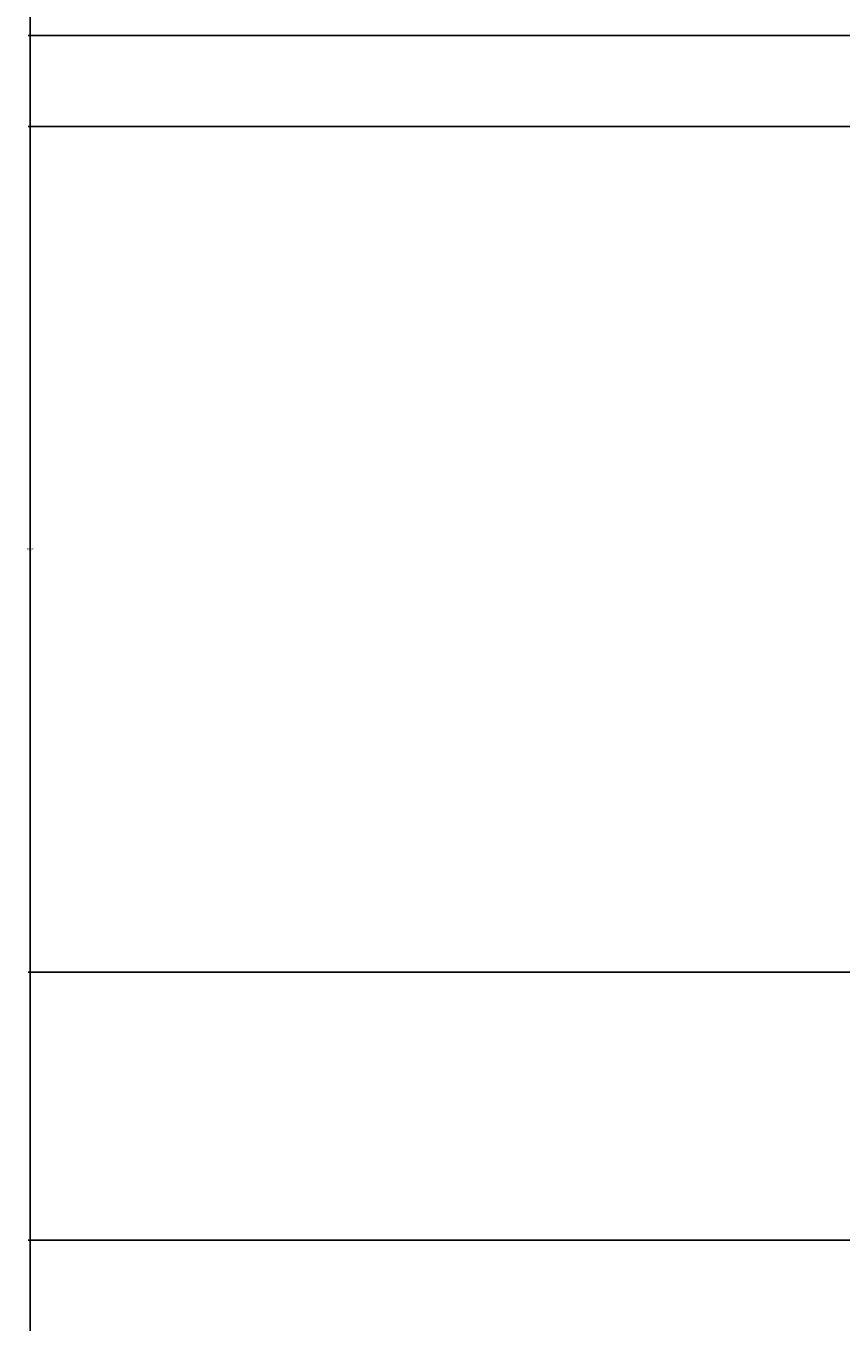
# Model space of a CAD drawing. Units: inches. Extents: x -61 to 1599, y -1316 to 257.
# Tile 56 of 204: x -61 to 12, y -282 to -166. Entities that reach past the tile are written whole.
import ezdxf

# ---------------------------------------------------------------- set-up
doc = ezdxf.new("R2010")
doc.units = ezdxf.units.IN
doc.header["$MEASUREMENT"] = 0
doc.layers.add('A-ANNO-DIMS', color=2, linetype='Continuous', lineweight=18)
doc.styles.get("Standard").update_dxf_attribs({"font": 'arial.ttf'})
doc.dimstyles.get("Standard").update_dxf_attribs({"dimtxt": 0.18, "dimasz": 0.18, "dimexe": 0.18, "dimexo": 0.0625, "dimgap": 0.09, "dimtad": 0, "dimtih": 1, "dimtoh": 1, "dimdec": 0, "dimzin": 0, "dimdsep": 46, "dimlunit": 3, "dimtxsty": 'Standard', "dimcen": 0.09, "dimadec": 0, "dimazin": 0, "dimtfac": 1, "dimtdec": 0, "dimtofl": 0, "dimtmove": 0, "dimatfit": 3, "dimfxl": 1, "dimtolj": 1, "dimtzin": 0, "dimarcsym": 0})

# ---------------------------------------------------------------- blocks, each defined once
blk = doc.blocks.new('*D687')
at = {"layer": 'A-ANNO-DIMS', "color": 0, "lineweight": -2, "transparency": 16777216}
for p, q in [((289.42, 181.68), (-61.08, 181.68)), ((-60.9, 181.5), (-60.9, -528.95)), ((-60.9, -1239.76), (-60.9, -529.32)), ((319.64, -1239.94), (-61.08, -1239.94))]:
    blk.add_line(p, q, dxfattribs=at)
at = {"layer": 'A-ANNO-DIMS', "color": 0, "transparency": 16777216}
for points in [[(-60.93, 181.5), (-60.87, 181.5), (-60.9, 181.68)], [(-60.93, -1239.76), (-60.87, -1239.76), (-60.9, -1239.94)]]:
    blk.add_solid(points, dxfattribs=at)
at = {"layer": 'DEFPOINTS', "color": 0, "transparency": 16777216}
for p in [(289.48, 181.68), (-60.9, -1239.94), (319.7, -1239.94)]:
    blk.add_point(p, dxfattribs=at)
at = {"layer": 'A-ANNO-DIMS', "color": 0, "transparency": 16777216, "insert": (-60.9, -529.13), "char_height": 0.18, "attachment_point": 5}
blk.add_mtext('\\A1;1421.6', dxfattribs=at)
blk = doc.blocks.new('*D691')
at = {"layer": 'A-ANNO-DIMS', "color": 0, "lineweight": -2, "transparency": 16777216}
for p, q in [((14.64, 157.68), (-61.08, 157.68)), ((-60.9, 157.5), (-60.9, -141.64)), ((-60.9, -441.14), (-60.9, -142)), ((14.64, -441.32), (-61.08, -441.32))]:
    blk.add_line(p, q, dxfattribs=at)
at = {"layer": 'A-ANNO-DIMS', "color": 0, "transparency": 16777216}
for points in [[(-60.93, 157.5), (-60.87, 157.5), (-60.9, 157.68)], [(-60.93, -441.14), (-60.87, -441.14), (-60.9, -441.32)]]:
    blk.add_solid(points, dxfattribs=at)
at = {"layer": 'DEFPOINTS', "color": 0, "transparency": 16777216}
for p in [(-60.9, 157.68), (14.7, 157.68), (14.7, -441.32)]:
    blk.add_point(p, dxfattribs=at)
at = {"layer": 'A-ANNO-DIMS', "color": 0, "transparency": 16777216, "insert": (-60.9, -141.82), "char_height": 0.18, "attachment_point": 5}
blk.add_mtext('\\A1;599', dxfattribs=at)
blk = doc.blocks.new('*D699')
at = {"layer": 'A-ANNO-DIMS', "color": 0, "lineweight": -2, "transparency": 16777216}
for p, q in [((835.64, -167.17), (-61.08, -167.17)), ((-60.9, -167.35), (-60.9, -306.73)), ((-60.9, -446.47), (-60.9, -307.09)), ((841.64, -446.65), (-61.08, -446.65))]:
    blk.add_line(p, q, dxfattribs=at)
at = {"layer": 'A-ANNO-DIMS', "color": 0, "transparency": 16777216}
for points in [[(-60.93, -167.35), (-60.87, -167.35), (-60.9, -167.17)], [(-60.93, -446.47), (-60.87, -446.47), (-60.9, -446.65)]]:
    blk.add_solid(points, dxfattribs=at)
at = {"layer": 'DEFPOINTS', "color": 0, "transparency": 16777216}
for p in [(835.7, -167.17), (-60.9, -446.65), (841.7, -446.65)]:
    blk.add_point(p, dxfattribs=at)
at = {"layer": 'A-ANNO-DIMS', "color": 0, "transparency": 16777216, "insert": (-60.9, -306.91), "char_height": 0.18, "attachment_point": 5}
blk.add_mtext('\\A1;279.5', dxfattribs=at)
blk = doc.blocks.new('*D706')
at = {"layer": 'A-ANNO-DIMS', "color": 0, "lineweight": -2, "transparency": 16777216}
for p, q in [((78.64, -175.32), (-61.08, -175.32)), ((-60.9, -175.5), (-60.9, -212.98)), ((-60.9, -250.81), (-60.9, -213.34)), ((78.64, -250.99), (-61.08, -250.99))]:
    blk.add_line(p, q, dxfattribs=at)
at = {"layer": 'A-ANNO-DIMS', "color": 0, "transparency": 16777216}
for points in [[(-60.93, -175.5), (-60.87, -175.5), (-60.9, -175.32)], [(-60.93, -250.81), (-60.87, -250.81), (-60.9, -250.99)]]:
    blk.add_solid(points, dxfattribs=at)
at = {"layer": 'DEFPOINTS', "color": 0, "transparency": 16777216}
for p in [(-60.9, -175.32), (78.7, -175.32), (78.7, -250.99)]:
    blk.add_point(p, dxfattribs=at)
at = {"layer": 'A-ANNO-DIMS', "color": 0, "transparency": 16777216, "insert": (-60.9, -213.16), "char_height": 0.18, "attachment_point": 5}
blk.add_mtext('\\A1;75.67', dxfattribs=at)
blk = doc.blocks.new('*D707')
at = {"layer": 'A-ANNO-DIMS', "color": 0, "lineweight": -2, "transparency": 16777216}
for p, q in [((78.64, -274.99), (-61.08, -274.99)), ((-60.9, -275.17), (-60.9, -308.47)), ((-60.9, -342.14), (-60.9, -308.84)), ((78.64, -342.32), (-61.08, -342.32))]:
    blk.add_line(p, q, dxfattribs=at)
at = {"layer": 'A-ANNO-DIMS', "color": 0, "transparency": 16777216}
for points in [[(-60.93, -275.17), (-60.87, -275.17), (-60.9, -274.99)], [(-60.93, -342.14), (-60.87, -342.14), (-60.9, -342.32)]]:
    blk.add_solid(points, dxfattribs=at)
at = {"layer": 'DEFPOINTS', "color": 0, "transparency": 16777216}
for p in [(78.7, -274.99), (-60.9, -342.32), (78.7, -342.32)]:
    blk.add_point(p, dxfattribs=at)
at = {"layer": 'A-ANNO-DIMS', "color": 0, "transparency": 16777216, "insert": (-60.9, -308.66), "char_height": 0.18, "attachment_point": 5}
blk.add_mtext('\\A1;67.33', dxfattribs=at)

msp = doc.modelspace()

# ---------------------------------------------------------------- dimensions: what is measured, and where the dimension line sits
at = {"layer": 'A-ANNO-DIMS'}
for base, p1, p2, override, picture, middle in [((-60.8972, -1239.9446), (289.4807, 181.6771), (319.7028, -1239.9446), {"dimdec": 1, "dimlfac": 1, "dimrnd": 0, "dimzin": 0, "dimdsep": 46, "dimlunit": 2}, '*D687', (-60.8972, -529.1337)), ((-60.8972, 157.6771), (14.7028, -441.3229), (14.7028, 157.6771), {"dimdec": 0, "dimlfac": 1, "dimrnd": 0, "dimzin": 0, "dimdsep": 46, "dimlunit": 2}, '*D691', (-60.8972, -141.8229)), ((-60.8972, -446.6462), (835.7028, -167.169), (841.7028, -446.6462), {"dimdec": 1, "dimlfac": 1, "dimrnd": 0, "dimzin": 0, "dimdsep": 46, "dimlunit": 2}, '*D699', (-60.8972, -306.9076)), ((-60.8972, -175.3229), (78.7028, -250.9938), (78.7028, -175.3229), {"dimdec": 2, "dimlfac": 1, "dimrnd": 0, "dimzin": 0, "dimdsep": 46, "dimlunit": 2}, '*D706', (-60.8972, -213.1583)), ((-60.8972, -342.3189), (78.7028, -274.9938), (78.7028, -342.3189), {"dimdec": 2, "dimlfac": 1, "dimrnd": 0, "dimzin": 0, "dimdsep": 46, "dimlunit": 2}, '*D707', (-60.8972, -308.6563))]:
    dim = msp.add_linear_dim(base=base, p1=p1, p2=p2, angle=90, dimstyle='Standard', override=override, dxfattribs=at)
    dim.commit()
    dim.dimension.update_dxf_attribs({"geometry": picture, "text_midpoint": middle})

doc.saveas('drawing.dxf')
